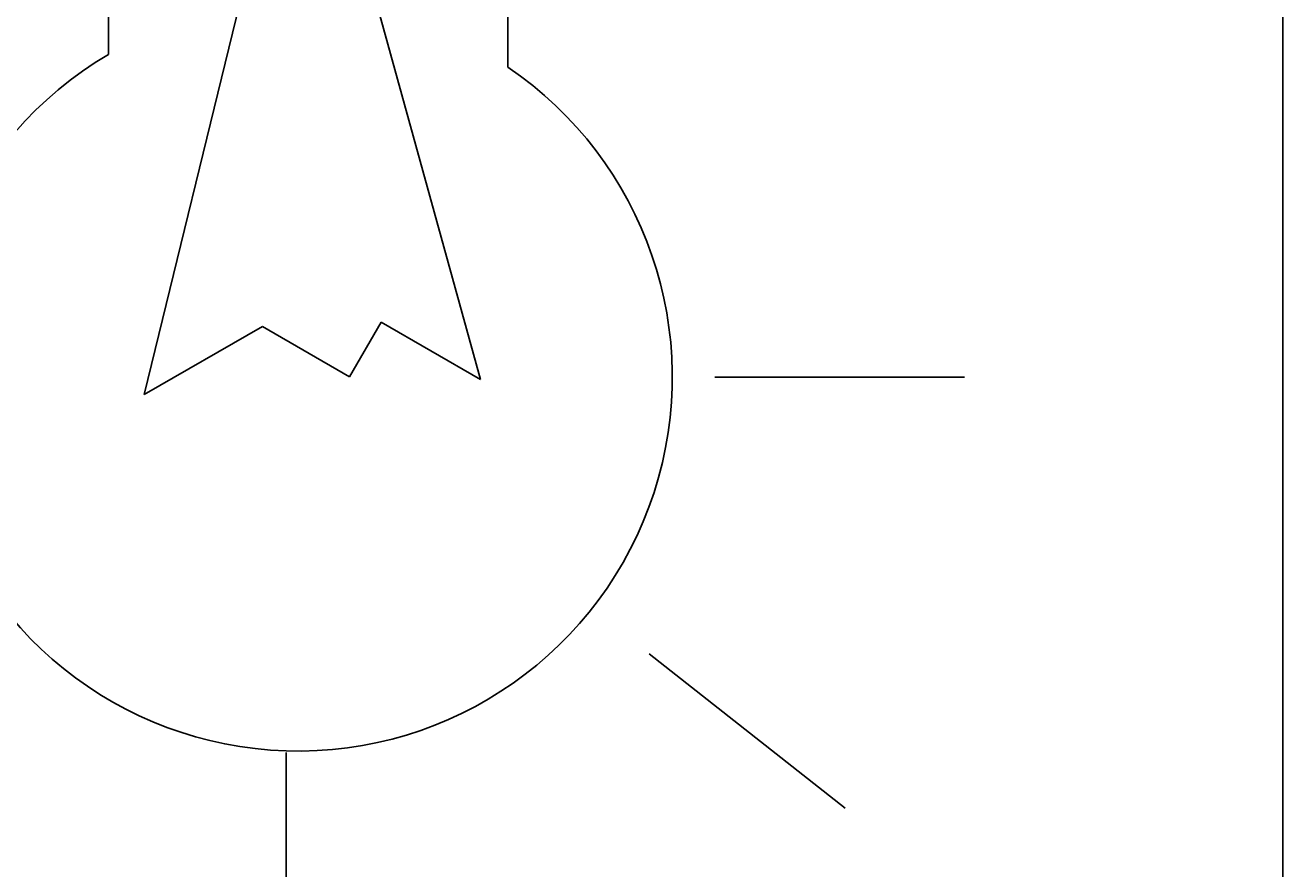
# Model space of a CAD drawing. Units: millimetres. Extents: x -8 to 285, y 5 to 221.
# Tile 28 of 30: x 221 to 271, y 132 to 166. Entities that reach past the tile are written whole.
import ezdxf

# ---------------------------------------------------------------- set-up
doc = ezdxf.new("R2010")
doc.units = ezdxf.units.MM
doc.layers.add('A-ANNO-DIMS', color=2, linetype='Continuous', lineweight=18)
doc.layers.add('E-LITE-FIXT', color=7, linetype='Continuous', lineweight=25)
doc.layers.add('E-POWR-AC-LINE', color=30, linetype='Continuous', lineweight=25, true_color=0xf26722)
doc.styles.get("Standard").update_dxf_attribs({"font": 'arial.ttf'})
doc.dimstyles.get("Standard").update_dxf_attribs({"dimtxt": 0.18, "dimasz": 0.18, "dimexe": 0.18, "dimexo": 0.0625, "dimgap": 0.09, "dimtad": 0, "dimtih": 1, "dimtoh": 1, "dimdec": 4, "dimzin": 0, "dimdsep": 46, "dimtxsty": 'Standard', "dimcen": 0.09, "dimadec": 0, "dimazin": 0, "dimtfac": 1, "dimtdec": 4, "dimtofl": 0, "dimtmove": 0, "dimatfit": 3, "dimfxl": 1, "dimtolj": 1, "dimtzin": 0, "dimarcsym": 0})

# ---------------------------------------------------------------- blocks, each defined once
blk = doc.blocks.new('LAMP-INCANDESCENT')
for p, q in [((7.407, 29.994), (10.595, 43.039)), ((23.407, 29.994), (18.595, 43.039)), ((9.734, 39.517), (19.894, 39.517)), ((9.001, 36.517), (21.001, 36.517)), ((8.268, 33.517), (22.107, 33.517)), ((7.407, 29.994), (7.407, 27.935)), ((12.666, 29.994), (8.834, 14.293)), ((22.321, 14.903), (18.146, 29.994)), ((23.407, 29.994), (23.407, 27.423)), ((17.067, 15.012), (18.333, 17.205)), ((18.333, 17.205), (22.321, 14.903)), ((8.834, 14.293), (13.574, 17.029)), ((13.574, 17.029), (17.067, 15.012))]:
    blk.add_line(p, q)
for points in [[(10.595, 43.039), (18.595, 43.039)], [(23.407, 29.994), (7.407, 29.994)]]:
    blk.add_lwpolyline(points)
for centre, radius, start, end in [((14.595, 43.039), 4, 0, 180), ((15.001, 15), 15, 88.4488, 91.5512), ((15.001, 15), 15, 120.4152, 55.9163)]:
    blk.add_arc(centre, radius, start, end)
blk = doc.blocks.new('*D9')
at = {"layer": 'A-ANNO-DIMS', "color": 0, "lineweight": -2, "transparency": 16777216}
for p, q in [((6.672, 133.79), (6.672, 220.737)), ((6.852, 220.557), (138.33, 220.557)), ((270.739, 220.557), (139.262, 220.557)), ((270.919, 206.519), (270.919, 220.737))]:
    blk.add_line(p, q, dxfattribs=at)
at = {"layer": 'A-ANNO-DIMS', "color": 0, "transparency": 16777216}
for points in [[(6.852, 220.587), (6.852, 220.527), (6.672, 220.557)], [(270.739, 220.587), (270.739, 220.527), (270.919, 220.557)]]:
    blk.add_solid(points, dxfattribs=at)
at = {"layer": 'Defpoints', "color": 0, "transparency": 16777216}
for p in [(270.919, 220.557), (270.919, 206.457), (6.672, 133.727)]:
    blk.add_point(p, dxfattribs=at)
at = {"layer": 'A-ANNO-DIMS', "color": 0, "transparency": 16777216, "insert": (138.796, 220.557), "char_height": 0.18, "attachment_point": 5}
blk.add_mtext('\\A1;264.25', dxfattribs=at)
blk = doc.blocks.new('*D14')
at = {"layer": 'A-ANNO-DIMS', "color": 0, "lineweight": -2, "transparency": 16777216}
for p, q in [((189.039, 137.013), (189.039, 5.222)), ((230.967, 137.013), (230.967, 5.222)), ((189.219, 5.402), (209.606, 5.402)), ((230.787, 5.402), (210.4, 5.402))]:
    blk.add_line(p, q, dxfattribs=at)
at = {"layer": 'A-ANNO-DIMS', "color": 0, "transparency": 16777216}
for points in [[(189.219, 5.432), (189.219, 5.372), (189.039, 5.402)], [(230.787, 5.432), (230.787, 5.372), (230.967, 5.402)]]:
    blk.add_solid(points, dxfattribs=at)
at = {"layer": 'Defpoints', "color": 0, "transparency": 16777216}
for p in [(189.039, 137.075), (230.967, 137.075), (230.967, 5.402)]:
    blk.add_point(p, dxfattribs=at)
at = {"layer": 'A-ANNO-DIMS', "color": 0, "transparency": 16777216, "insert": (210.003, 5.402), "char_height": 0.18, "attachment_point": 5}
blk.add_mtext('\\A1;41.93', dxfattribs=at)

msp = doc.modelspace()

# ---------------------------------------------------------------- linework, layer by layer
at = {"layer": 'E-LITE-FIXT'}
for p, q in [((258.1552, 152.0675), (248.1552, 152.0675)), ((245.5173, 140.9643), (253.3748, 134.7789))]:
    msp.add_line(p, q, dxfattribs=at)
at = {"layer": 'E-POWR-AC-LINE'}
msp.add_lwpolyline([(244.6186, 34.6512), (244.6186, 49.925), (270.9192, 49.925), (270.9192, 206.4568), (145.1651, 206.4568), (145.1651, 201.7939)], dxfattribs=at)

# ---------------------------------------------------------------- block references
at = {"layer": 'E-LITE-FIXT'}
msp.add_blockref('LAMP-INCANDESCENT', (216.4466, 137.068), dxfattribs=at)

# ---------------------------------------------------------------- dimensions: what is measured, and where the dimension line sits
at = {"layer": 'A-ANNO-DIMS'}
for base, p1, p2, picture, middle in [((270.9192, 220.5568), (6.6725, 133.7273), (270.9192, 206.4568), '*D9', (138.7958, 220.5568)), ((230.9672, 5.402), (189.039, 137.0752), (230.9672, 137.0752), '*D14', (210.0031, 5.402))]:
    dim = msp.add_linear_dim(base=base, p1=p1, p2=p2, dimstyle='Standard', override={"dimdec": 2, "dimlfac": 1, "dimrnd": 0, "dimzin": 0, "dimdsep": 46, "dimlunit": 2}, dxfattribs=at)
    dim.commit()
    dim.dimension.update_dxf_attribs({"geometry": picture, "text_midpoint": middle})

doc.saveas('drawing.dxf')
